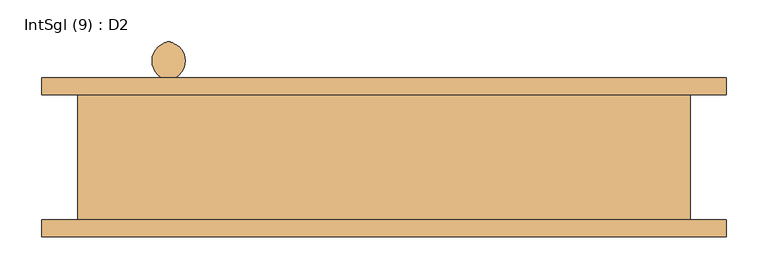
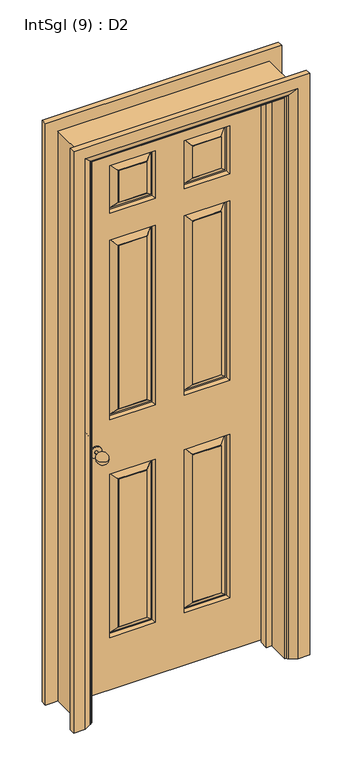
"""IFC4 building model written with IfcOpenShell, lengths in millimetres: door geometry, IntSgl (9) : D2."""

from ifc_helpers import new_model, si_unit, point, frame, origin, place, context, project, spatial, polyline, circle_curve, ellipse_curve, trimmed, outline, extrude, faceted_brep, source, transform, mapped, element, save
from ifc_brep_helpers import plane_surface, cylinder_surface, revolved_surface, advanced_brep


def intsgl_9_d2_8283ee4d(model_context):
    return source(origin(), model_context, "Body", "SolidModel", [
        advanced_brep(
        [(-253.0, 18.0, 900.0), (-258.0, -26.437411, 900.0), (-263.0, 18.0, 900.0), (-263.0, 33.0, 900.0), (-253.0, 33.0, 900.0), (-278.0, 37.0, 900.0), (-238.0, 37.0, 900.0), (-278.0, 33.0, 900.0), (-238.0, 33.0, 900.0)],
        [
            (0, 1, circle_curve(frame((-261.1884862, -3.5786495, 900.0), z_axis=(0.0, 0.0, -1.0), x_axis=(0.0, 1.0, 0.0)), 23.0800654)),
            (1, 2, circle_curve(frame((-254.8115138, -3.5786495, 900.0), z_axis=(0.0, 0.0, -1.0), x_axis=(0.0, 1.0, 0.0)), 23.0800654)),
            (2, 0, circle_curve(frame((-258.0, 18.0, 900.0), z_axis=(0.0, -1.0, 0.0), x_axis=(-1.0, 0.0, 0.0)), 5.0)),
            (0, 2, circle_curve(frame((-258.0, 18.0, 900.0), z_axis=(0.0, -1.0, 0.0), x_axis=(-1.0, 0.0, 0.0)), 5.0)),
            (2, 3),
            (3, 4, circle_curve(frame((-258.0, 33.0, 900.0), z_axis=(0.0, -1.0, 0.0), x_axis=(-1.0, 0.0, 0.0)), 5.0)),
            (4, 0),
            (4, 3, circle_curve(frame((-258.0, 33.0, 900.0), z_axis=(0.0, -1.0, 0.0), x_axis=(-1.0, 0.0, 0.0)), 5.0)),
            (5, 6, circle_curve(frame((-258.0, 37.0, 900.0), z_axis=(0.0, 1.0, 0.0), x_axis=(1.0, 0.0, 0.0)), 20.0)),
            (6, 5, circle_curve(frame((-258.0, 37.0, 900.0), z_axis=(0.0, 1.0, 0.0), x_axis=(1.0, 0.0, 0.0)), 20.0)),
            (7, 8, circle_curve(frame((-258.0, 33.0, 900.0), z_axis=(0.0, -1.0, 0.0), x_axis=(1.0, 0.0, 0.0)), 20.0)),
            (8, 7, circle_curve(frame((-258.0, 33.0, 900.0), z_axis=(0.0, -1.0, 0.0), x_axis=(1.0, 0.0, 0.0)), 20.0)),
            (6, 8),
            (7, 5),
        ],
        [
            revolved_surface(trimmed(ellipse_curve(frame((-254.8115138, -3.5786495, 900.0), z_axis=(0.0, 0.0, -1.0), x_axis=(0.0, 1.0, 0.0)), 23.0800654, 23.0800654), [point((-258.0, -26.437411, 900.0))], [point((-263.0, 18.0, 900.0))], True, "CARTESIAN"), (-258.0, 33.0, 900.0), (0.0, 1.0, 0.0)),
            cylinder_surface(frame((-258.0, 33.0, 900.0), z_axis=(0.0, 1.0, 0.0), x_axis=(-1.0, 0.0, 0.0)), 5.0),
            plane_surface(frame((-238.0, 37.0, 900.0), z_axis=(0.0, 1.0, 0.0), x_axis=(0.0, 0.0, 1.0))),
            plane_surface(frame((-238.0, 33.0, 900.0), z_axis=(0.0, -1.0, 0.0), x_axis=(0.0, 0.0, -1.0))),
            cylinder_surface(frame((-258.0, 33.0, 900.0), z_axis=(0.0, 1.0, 0.0), x_axis=(1.0, 0.0, 0.0)), 20.0),
        ],
        [
            (0, [[1, 2, 3]]),
            (0, [[-1, 4, -2]]),
            (1, [[5, 6, 7, -3]]),
            (1, [[-7, 8, -5, -4]]),
            (2, [[9, 10]]),
            (3, [[11, 12], [-8, -6]]),
            (4, [[13, -11, 14, -10]]),
            (4, [[-14, -12, -13, -9]]),
        ],
    ),
        advanced_brep(
        [(-253.0, 94.0, 900.0), (-263.0, 94.0, 900.0), (-258.0, 138.437411, 900.0), (-253.0, 79.0, 900.0), (-263.0, 79.0, 900.0), (-278.0, 75.0, 900.0), (-238.0, 75.0, 900.0), (-278.0, 79.0, 900.0), (-238.0, 79.0, 900.0)],
        [
            (0, 1, circle_curve(frame((-258.0, 94.0, 900.0), z_axis=(0.0, 1.0, 0.0), x_axis=(-1.0, 0.0, 0.0)), 5.0)),
            (1, 2, circle_curve(frame((-254.8115138, 115.5786495, 900.0), z_axis=(0.0, 0.0, -1.0), x_axis=(0.0, -1.0, 0.0)), 23.0800654)),
            (2, 0, circle_curve(frame((-261.1884862, 115.5786495, 900.0), z_axis=(0.0, 0.0, -1.0), x_axis=(0.0, -1.0, 0.0)), 23.0800654)),
            (1, 0, circle_curve(frame((-258.0, 94.0, 900.0), z_axis=(0.0, 1.0, 0.0), x_axis=(-1.0, 0.0, 0.0)), 5.0)),
            (0, 3),
            (3, 4, circle_curve(frame((-258.0, 79.0, 900.0), z_axis=(0.0, 1.0, 0.0), x_axis=(-1.0, 0.0, 0.0)), 5.0)),
            (4, 1),
            (4, 3, circle_curve(frame((-258.0, 79.0, 900.0), z_axis=(0.0, 1.0, 0.0), x_axis=(-1.0, 0.0, 0.0)), 5.0)),
            (5, 6, circle_curve(frame((-258.0, 75.0, 900.0), z_axis=(0.0, -1.0, 0.0), x_axis=(1.0, 0.0, 0.0)), 20.0)),
            (6, 5, circle_curve(frame((-258.0, 75.0, 900.0), z_axis=(0.0, -1.0, 0.0), x_axis=(1.0, 0.0, 0.0)), 20.0)),
            (7, 8, circle_curve(frame((-258.0, 79.0, 900.0), z_axis=(0.0, 1.0, 0.0), x_axis=(1.0, 0.0, 0.0)), 20.0)),
            (8, 7, circle_curve(frame((-258.0, 79.0, 900.0), z_axis=(0.0, 1.0, 0.0), x_axis=(1.0, 0.0, 0.0)), 20.0)),
            (5, 7),
            (8, 6),
        ],
        [
            revolved_surface(trimmed(ellipse_curve(frame((-254.8115138, 115.5786495, 900.0), z_axis=(0.0, 0.0, 1.0), x_axis=(0.0, -1.0, 0.0)), 23.0800654, 23.0800654), [point((-258.0, 138.437411, 900.0))], [point((-263.0, 94.0, 900.0))], True, "CARTESIAN"), (-258.0, 79.0, 900.0), (0.0, -1.0, 0.0)),
            cylinder_surface(frame((-258.0, 79.0, 900.0), z_axis=(0.0, -1.0, 0.0), x_axis=(-1.0, 0.0, 0.0)), 5.0),
            plane_surface(frame((-238.0, 75.0, 900.0), z_axis=(0.0, -1.0, 0.0), x_axis=(0.0, 0.0, 1.0))),
            plane_surface(frame((-238.0, 79.0, 900.0), z_axis=(0.0, 1.0, 0.0), x_axis=(0.0, 0.0, -1.0))),
            cylinder_surface(frame((-258.0, 79.0, 900.0), z_axis=(0.0, -1.0, 0.0), x_axis=(1.0, 0.0, 0.0)), 20.0),
        ],
        [
            (0, [[1, 2, 3]]),
            (0, [[-2, 4, -3]]),
            (1, [[-1, 5, 6, 7]]),
            (1, [[-4, -7, 8, -5]]),
            (2, [[9, 10]]),
            (3, [[11, 12], [-6, -8]]),
            (4, [[-9, 13, -12, 14]]),
            (4, [[-10, -14, -11, -13]]),
        ],
    ),
        faceted_brep([(-333.0, 37.0, 2058.0), (-333.0, 37.0, 8.0), (333.0, 37.0, 8.0), (333.0, 37.0, 2058.0), (-50.0, 37.0, 800.0), (-50.0, 37.0, 200.0), (-208.0, 37.0, 200.0), (-208.0, 37.0, 800.0), (208.0, 37.0, 800.0), (208.0, 37.0, 200.0), (50.0, 37.0, 200.0), (50.0, 37.0, 800.0), (-50.0, 37.0, 1658.0), (-50.0, 37.0, 1000.0), (-208.0, 37.0, 1000.0), (-208.0, 37.0, 1658.0), (208.0, 37.0, 1658.0), (208.0, 37.0, 1000.0), (50.0, 37.0, 1000.0), (50.0, 37.0, 1658.0), (-50.0, 37.0, 1933.0), (-50.0, 37.0, 1758.0), (-208.0, 37.0, 1758.0), (-208.0, 37.0, 1933.0), (208.0, 37.0, 1933.0), (208.0, 37.0, 1758.0), (50.0, 37.0, 1758.0), (50.0, 37.0, 1933.0), (-80.0, 37.0, 230.0), (-80.0, 37.0, 770.0), (-178.0, 37.0, 770.0), (-178.0, 37.0, 230.0), (178.0, 37.0, 230.0), (178.0, 37.0, 770.0), (80.0, 37.0, 770.0), (80.0, 37.0, 230.0), (-80.0, 37.0, 1030.0), (-80.0, 37.0, 1628.0), (-178.0, 37.0, 1628.0), (-178.0, 37.0, 1030.0), (178.0, 37.0, 1030.0), (178.0, 37.0, 1628.0), (80.0, 37.0, 1628.0), (80.0, 37.0, 1030.0), (-80.0, 37.0, 1788.0), (-80.0, 37.0, 1903.0), (-178.0, 37.0, 1903.0), (-178.0, 37.0, 1788.0), (178.0, 37.0, 1788.0), (178.0, 37.0, 1903.0), (80.0, 37.0, 1903.0), (80.0, 37.0, 1788.0), (-333.0, 75.0, 2058.0), (333.0, 75.0, 2058.0), (333.0, 75.0, 8.0), (-333.0, 75.0, 8.0), (50.0, 75.0, 800.0), (50.0, 75.0, 200.0), (208.0, 75.0, 200.0), (208.0, 75.0, 800.0), (-208.0, 75.0, 800.0), (-208.0, 75.0, 200.0), (-50.0, 75.0, 200.0), (-50.0, 75.0, 800.0), (50.0, 75.0, 1658.0), (50.0, 75.0, 1000.0), (208.0, 75.0, 1000.0), (208.0, 75.0, 1658.0), (-208.0, 75.0, 1658.0), (-208.0, 75.0, 1000.0), (-50.0, 75.0, 1000.0), (-50.0, 75.0, 1658.0), (50.0, 75.0, 1933.0), (50.0, 75.0, 1758.0), (208.0, 75.0, 1758.0), (208.0, 75.0, 1933.0), (-208.0, 75.0, 1933.0), (-208.0, 75.0, 1758.0), (-50.0, 75.0, 1758.0), (-50.0, 75.0, 1933.0), (80.0, 75.0, 230.0), (80.0, 75.0, 770.0), (178.0, 75.0, 770.0), (178.0, 75.0, 230.0), (-178.0, 75.0, 230.0), (-178.0, 75.0, 770.0), (-80.0, 75.0, 770.0), (-80.0, 75.0, 230.0), (80.0, 75.0, 1030.0), (80.0, 75.0, 1628.0), (178.0, 75.0, 1628.0), (178.0, 75.0, 1030.0), (-178.0, 75.0, 1030.0), (-178.0, 75.0, 1628.0), (-80.0, 75.0, 1628.0), (-80.0, 75.0, 1030.0), (80.0, 75.0, 1788.0), (80.0, 75.0, 1903.0), (178.0, 75.0, 1903.0), (178.0, 75.0, 1788.0), (-178.0, 75.0, 1788.0), (-178.0, 75.0, 1903.0), (-80.0, 75.0, 1903.0), (-80.0, 75.0, 1788.0), (80.0, 74.0, 230.0), (80.0, 74.0, 770.0), (58.0, 60.0, 208.0), (58.0, 60.0, 792.0), (78.0, 74.0, 772.0), (78.0, 74.0, 228.0), (53.0, 60.0, 797.0), (53.0, 60.0, 203.0), (178.0, 74.0, 770.0), (200.0, 60.0, 792.0), (180.0, 74.0, 772.0), (205.0, 60.0, 797.0), (178.0, 74.0, 230.0), (200.0, 60.0, 208.0), (180.0, 74.0, 228.0), (205.0, 60.0, 203.0), (-178.0, 74.0, 230.0), (-178.0, 74.0, 770.0), (-200.0, 60.0, 208.0), (-200.0, 60.0, 792.0), (-180.0, 74.0, 772.0), (-180.0, 74.0, 228.0), (-205.0, 60.0, 797.0), (-205.0, 60.0, 203.0), (-80.0, 74.0, 770.0), (-58.0, 60.0, 792.0), (-78.0, 74.0, 772.0), (-53.0, 60.0, 797.0), (-80.0, 74.0, 230.0), (-58.0, 60.0, 208.0), (-78.0, 74.0, 228.0), (-53.0, 60.0, 203.0), (80.0, 74.0, 1030.0), (80.0, 74.0, 1628.0), (58.0, 60.0, 1008.0), (58.0, 60.0, 1650.0), (78.0, 74.0, 1630.0), (78.0, 74.0, 1028.0), (53.0, 60.0, 1655.0), (53.0, 60.0, 1003.0), (178.0, 74.0, 1628.0), (200.0, 60.0, 1650.0), (180.0, 74.0, 1630.0), (205.0, 60.0, 1655.0), (178.0, 74.0, 1030.0), (200.0, 60.0, 1008.0), (180.0, 74.0, 1028.0), (205.0, 60.0, 1003.0), (-178.0, 74.0, 1030.0), (-178.0, 74.0, 1628.0), (-200.0, 60.0, 1008.0), (-200.0, 60.0, 1650.0), (-180.0, 74.0, 1630.0), (-180.0, 74.0, 1028.0), (-205.0, 60.0, 1655.0), (-205.0, 60.0, 1003.0), (-80.0, 74.0, 1628.0), (-58.0, 60.0, 1650.0), (-78.0, 74.0, 1630.0), (-53.0, 60.0, 1655.0), (-80.0, 74.0, 1030.0), (-58.0, 60.0, 1008.0), (-78.0, 74.0, 1028.0), (-53.0, 60.0, 1003.0), (80.0, 74.0, 1788.0), (80.0, 74.0, 1903.0), (58.0, 60.0, 1766.0), (58.0, 60.0, 1925.0), (78.0, 74.0, 1905.0), (78.0, 74.0, 1786.0), (53.0, 60.0, 1930.0), (53.0, 60.0, 1761.0), (178.0, 74.0, 1903.0), (200.0, 60.0, 1925.0), (180.0, 74.0, 1905.0), (205.0, 60.0, 1930.0), (178.0, 74.0, 1788.0), (200.0, 60.0, 1766.0), (180.0, 74.0, 1786.0), (205.0, 60.0, 1761.0), (-178.0, 74.0, 1788.0), (-178.0, 74.0, 1903.0), (-200.0, 60.0, 1766.0), (-200.0, 60.0, 1925.0), (-180.0, 74.0, 1905.0), (-180.0, 74.0, 1786.0), (-205.0, 60.0, 1930.0), (-205.0, 60.0, 1761.0), (-80.0, 74.0, 1903.0), (-58.0, 60.0, 1925.0), (-78.0, 74.0, 1905.0), (-53.0, 60.0, 1930.0), (-80.0, 74.0, 1788.0), (-58.0, 60.0, 1766.0), (-78.0, 74.0, 1786.0), (-53.0, 60.0, 1761.0), (-80.0, 38.0, 230.0), (-80.0, 38.0, 770.0), (-58.0, 52.0, 208.0), (-58.0, 52.0, 792.0), (-78.0, 38.0, 772.0), (-78.0, 38.0, 228.0), (-53.0, 52.0, 797.0), (-53.0, 52.0, 203.0), (-178.0, 38.0, 770.0), (-200.0, 52.0, 792.0), (-180.0, 38.0, 772.0), (-205.0, 52.0, 797.0), (-178.0, 38.0, 230.0), (-200.0, 52.0, 208.0), (-180.0, 38.0, 228.0), (-205.0, 52.0, 203.0), (178.0, 38.0, 230.0), (178.0, 38.0, 770.0), (200.0, 52.0, 208.0), (200.0, 52.0, 792.0), (180.0, 38.0, 772.0), (180.0, 38.0, 228.0), (205.0, 52.0, 797.0), (205.0, 52.0, 203.0), (80.0, 38.0, 770.0), (58.0, 52.0, 792.0), (78.0, 38.0, 772.0), (53.0, 52.0, 797.0), (80.0, 38.0, 230.0), (58.0, 52.0, 208.0), (78.0, 38.0, 228.0), (53.0, 52.0, 203.0), (-80.0, 38.0, 1030.0), (-80.0, 38.0, 1628.0), (-58.0, 52.0, 1008.0), (-58.0, 52.0, 1650.0), (-78.0, 38.0, 1630.0), (-78.0, 38.0, 1028.0), (-53.0, 52.0, 1655.0), (-53.0, 52.0, 1003.0), (-178.0, 38.0, 1628.0), (-200.0, 52.0, 1650.0), (-180.0, 38.0, 1630.0), (-205.0, 52.0, 1655.0), (-178.0, 38.0, 1030.0), (-200.0, 52.0, 1008.0), (-180.0, 38.0, 1028.0), (-205.0, 52.0, 1003.0), (178.0, 38.0, 1030.0), (178.0, 38.0, 1628.0), (200.0, 52.0, 1008.0), (200.0, 52.0, 1650.0), (180.0, 38.0, 1630.0), (180.0, 38.0, 1028.0), (205.0, 52.0, 1655.0), (205.0, 52.0, 1003.0), (80.0, 38.0, 1628.0), (58.0, 52.0, 1650.0), (78.0, 38.0, 1630.0), (53.0, 52.0, 1655.0), (80.0, 38.0, 1030.0), (58.0, 52.0, 1008.0), (78.0, 38.0, 1028.0), (53.0, 52.0, 1003.0), (-80.0, 38.0, 1788.0), (-80.0, 38.0, 1903.0), (-58.0, 52.0, 1766.0), (-58.0, 52.0, 1925.0), (-78.0, 38.0, 1905.0), (-78.0, 38.0, 1786.0), (-53.0, 52.0, 1930.0), (-53.0, 52.0, 1761.0), (-178.0, 38.0, 1903.0), (-200.0, 52.0, 1925.0), (-180.0, 38.0, 1905.0), (-205.0, 52.0, 1930.0), (-178.0, 38.0, 1788.0), (-200.0, 52.0, 1766.0), (-180.0, 38.0, 1786.0), (-205.0, 52.0, 1761.0), (178.0, 38.0, 1788.0), (178.0, 38.0, 1903.0), (200.0, 52.0, 1766.0), (200.0, 52.0, 1925.0), (180.0, 38.0, 1905.0), (180.0, 38.0, 1786.0), (205.0, 52.0, 1930.0), (205.0, 52.0, 1761.0), (80.0, 38.0, 1903.0), (58.0, 52.0, 1925.0), (78.0, 38.0, 1905.0), (53.0, 52.0, 1930.0), (80.0, 38.0, 1788.0), (58.0, 52.0, 1766.0), (78.0, 38.0, 1786.0), (53.0, 52.0, 1761.0)], [[[0, 1, 2, 3], [4, 5, 6, 7], [8, 9, 10, 11], [12, 13, 14, 15], [16, 17, 18, 19], [20, 21, 22, 23], [24, 25, 26, 27]], [[28, 29, 30, 31]], [[32, 33, 34, 35]], [[36, 37, 38, 39]], [[40, 41, 42, 43]], [[44, 45, 46, 47]], [[48, 49, 50, 51]], [[52, 53, 54, 55], [56, 57, 58, 59], [60, 61, 62, 63], [64, 65, 66, 67], [68, 69, 70, 71], [72, 73, 74, 75], [76, 77, 78, 79]], [[80, 81, 82, 83]], [[84, 85, 86, 87]], [[88, 89, 90, 91]], [[92, 93, 94, 95]], [[96, 97, 98, 99]], [[100, 101, 102, 103]], [[1, 0, 52, 55]], [[2, 1, 55, 54]], [[3, 2, 54, 53]], [[0, 3, 53, 52]], [[104, 105, 81, 80]], [[106, 107, 108, 109]], [[56, 110, 111, 57]], [[81, 105, 112, 82]], [[108, 107, 113, 114]], [[110, 56, 59, 115]], [[82, 112, 116, 83]], [[114, 113, 117, 118]], [[115, 59, 58, 119]], [[104, 80, 83, 116]], [[109, 108, 114, 118], [105, 104, 116, 112]], [[106, 109, 118, 117]], [[111, 110, 115, 119], [107, 106, 117, 113]], [[57, 111, 119, 58]], [[120, 121, 85, 84]], [[122, 123, 124, 125]], [[60, 126, 127, 61]], [[85, 121, 128, 86]], [[124, 123, 129, 130]], [[126, 60, 63, 131]], [[86, 128, 132, 87]], [[130, 129, 133, 134]], [[131, 63, 62, 135]], [[120, 84, 87, 132]], [[125, 124, 130, 134], [121, 120, 132, 128]], [[122, 125, 134, 133]], [[127, 126, 131, 135], [123, 122, 133, 129]], [[61, 127, 135, 62]], [[136, 137, 89, 88]], [[138, 139, 140, 141]], [[64, 142, 143, 65]], [[89, 137, 144, 90]], [[140, 139, 145, 146]], [[142, 64, 67, 147]], [[90, 144, 148, 91]], [[146, 145, 149, 150]], [[147, 67, 66, 151]], [[136, 88, 91, 148]], [[141, 140, 146, 150], [137, 136, 148, 144]], [[138, 141, 150, 149]], [[143, 142, 147, 151], [139, 138, 149, 145]], [[65, 143, 151, 66]], [[152, 153, 93, 92]], [[154, 155, 156, 157]], [[68, 158, 159, 69]], [[93, 153, 160, 94]], [[156, 155, 161, 162]], [[158, 68, 71, 163]], [[94, 160, 164, 95]], [[162, 161, 165, 166]], [[163, 71, 70, 167]], [[152, 92, 95, 164]], [[157, 156, 162, 166], [153, 152, 164, 160]], [[154, 157, 166, 165]], [[159, 158, 163, 167], [155, 154, 165, 161]], [[69, 159, 167, 70]], [[168, 169, 97, 96]], [[170, 171, 172, 173]], [[72, 174, 175, 73]], [[97, 169, 176, 98]], [[172, 171, 177, 178]], [[174, 72, 75, 179]], [[98, 176, 180, 99]], [[178, 177, 181, 182]], [[179, 75, 74, 183]], [[168, 96, 99, 180]], [[173, 172, 178, 182], [169, 168, 180, 176]], [[170, 173, 182, 181]], [[175, 174, 179, 183], [171, 170, 181, 177]], [[73, 175, 183, 74]], [[184, 185, 101, 100]], [[186, 187, 188, 189]], [[76, 190, 191, 77]], [[101, 185, 192, 102]], [[188, 187, 193, 194]], [[190, 76, 79, 195]], [[102, 192, 196, 103]], [[194, 193, 197, 198]], [[195, 79, 78, 199]], [[184, 100, 103, 196]], [[189, 188, 194, 198], [185, 184, 196, 192]], [[186, 189, 198, 197]], [[191, 190, 195, 199], [187, 186, 197, 193]], [[77, 191, 199, 78]], [[200, 201, 29, 28]], [[202, 203, 204, 205]], [[4, 206, 207, 5]], [[29, 201, 208, 30]], [[204, 203, 209, 210]], [[206, 4, 7, 211]], [[30, 208, 212, 31]], [[210, 209, 213, 214]], [[211, 7, 6, 215]], [[200, 28, 31, 212]], [[205, 204, 210, 214], [201, 200, 212, 208]], [[202, 205, 214, 213]], [[207, 206, 211, 215], [203, 202, 213, 209]], [[5, 207, 215, 6]], [[216, 217, 33, 32]], [[218, 219, 220, 221]], [[8, 222, 223, 9]], [[33, 217, 224, 34]], [[220, 219, 225, 226]], [[222, 8, 11, 227]], [[34, 224, 228, 35]], [[226, 225, 229, 230]], [[227, 11, 10, 231]], [[216, 32, 35, 228]], [[221, 220, 226, 230], [217, 216, 228, 224]], [[218, 221, 230, 229]], [[223, 222, 227, 231], [219, 218, 229, 225]], [[9, 223, 231, 10]], [[232, 233, 37, 36]], [[234, 235, 236, 237]], [[12, 238, 239, 13]], [[37, 233, 240, 38]], [[236, 235, 241, 242]], [[238, 12, 15, 243]], [[38, 240, 244, 39]], [[242, 241, 245, 246]], [[243, 15, 14, 247]], [[232, 36, 39, 244]], [[237, 236, 242, 246], [233, 232, 244, 240]], [[234, 237, 246, 245]], [[239, 238, 243, 247], [235, 234, 245, 241]], [[13, 239, 247, 14]], [[248, 249, 41, 40]], [[250, 251, 252, 253]], [[16, 254, 255, 17]], [[41, 249, 256, 42]], [[252, 251, 257, 258]], [[254, 16, 19, 259]], [[42, 256, 260, 43]], [[258, 257, 261, 262]], [[259, 19, 18, 263]], [[248, 40, 43, 260]], [[253, 252, 258, 262], [249, 248, 260, 256]], [[250, 253, 262, 261]], [[255, 254, 259, 263], [251, 250, 261, 257]], [[17, 255, 263, 18]], [[264, 265, 45, 44]], [[266, 267, 268, 269]], [[20, 270, 271, 21]], [[45, 265, 272, 46]], [[268, 267, 273, 274]], [[270, 20, 23, 275]], [[46, 272, 276, 47]], [[274, 273, 277, 278]], [[275, 23, 22, 279]], [[264, 44, 47, 276]], [[269, 268, 274, 278], [265, 264, 276, 272]], [[266, 269, 278, 277]], [[271, 270, 275, 279], [267, 266, 277, 273]], [[21, 271, 279, 22]], [[280, 281, 49, 48]], [[282, 283, 284, 285]], [[24, 286, 287, 25]], [[49, 281, 288, 50]], [[284, 283, 289, 290]], [[286, 24, 27, 291]], [[50, 288, 292, 51]], [[290, 289, 293, 294]], [[291, 27, 26, 295]], [[280, 48, 51, 292]], [[285, 284, 290, 294], [281, 280, 292, 288]], [[282, 285, 294, 293]], [[287, 286, 291, 295], [283, 282, 293, 289]], [[25, 287, 295, 26]]]),
        faceted_brep([(-335.0, 75.0, 0.0), (-335.0, -75.0, 0.0), (-367.0, -75.0, 0.0), (-367.0, 75.0, 0.0), (-335.0, 75.0, 2060.0), (-335.0, -75.0, 2060.0), (-367.0, -75.0, 2092.0), (-367.0, 75.0, 2092.0), (335.0, 75.0, 0.0), (367.0, 75.0, 0.0), (367.0, -75.0, 0.0), (335.0, -75.0, 0.0), (335.0, 75.0, 2060.0), (367.0, 75.0, 2092.0), (367.0, -75.0, 2092.0), (335.0, -75.0, 2060.0)], [[[0, 1, 2, 3]], [[1, 0, 4, 5]], [[2, 1, 5, 6]], [[3, 2, 6, 7]], [[0, 3, 7, 4]], [[8, 9, 10, 11]], [[12, 13, 9, 8]], [[13, 14, 10, 9]], [[14, 15, 11, 10]], [[15, 12, 8, 11]], [[5, 4, 12, 15]], [[6, 5, 15, 14]], [[7, 6, 14, 13]], [[4, 7, 13, 12]]]),
        extrude(outline(polyline([(0.0, -335.0), (0.0, -316.0), (2041.0, -316.0), (2041.0, 316.0), (0.0, 316.0), (0.0, 335.0), (2060.0, 335.0), (2060.0, -335.0), (0.0, -335.0)])), frame((0.0, 3.0, 0.0), z_axis=(0.0, 1.0, 0.0), x_axis=(0.0, 0.0, 1.0)), (0.0, 0.0, 1.0), 32.0),
        advanced_brep(
        [(-410.0, -95.0, 0.0), (-410.0, -75.0, 0.0), (-340.0, -75.0, 0.0), (-344.0, -81.0, 0.0), (-370.0, -95.0, 0.0), (-410.0, -95.0, 2135.0), (-410.0, -75.0, 2135.0), (410.0, -75.0, 2135.0), (410.0, -75.0, 0.0), (340.0, -75.0, 0.0), (340.0, -75.0, 2065.0), (-340.0, -75.0, 2065.0), (-344.0, -81.0, 2069.0), (-370.0, -95.0, 2095.0), (370.0, -95.0, 2095.0), (370.0, -95.0, 0.0), (410.0, -95.0, 0.0), (410.0, -95.0, 2135.0), (344.0, -81.0, 0.0), (344.0, -81.0, 2069.0)],
        [
            (0, 1),
            (1, 2),
            (2, 3, circle_curve(frame((-348.0, -74.0, 0.0), z_axis=(0.0, 0.0, -1.0), x_axis=(-1.0, 0.0, 0.0)), 8.0622577)),
            (3, 4),
            (4, 0),
            (0, 5),
            (5, 6),
            (6, 1),
            (6, 7),
            (7, 8),
            (8, 9),
            (9, 10),
            (10, 11),
            (11, 2),
            (11, 12, ellipse_curve(frame((-348.0, -74.0, 2073.0), z_axis=(-0.7071067811865475, 0.0, -0.7071067811865475), x_axis=(0.7071067811865474, 0.0, -0.7071067811865476)), 11.4017543, 8.0622577)),
            (12, 3),
            (12, 13),
            (13, 4),
            (13, 14),
            (14, 15),
            (15, 16),
            (16, 17),
            (17, 5),
            (7, 17),
            (16, 8),
            (15, 18),
            (18, 9, circle_curve(frame((348.0, -74.0, 0.0), z_axis=(0.0, 0.0, -1.0), x_axis=(1.0, 0.0, 0.0)), 8.0622577)),
            (19, 10, ellipse_curve(frame((348.0, -74.0, 2073.0), z_axis=(0.7071067811865475, 0.0, -0.7071067811865475), x_axis=(0.7071067811865474, 0.0, 0.7071067811865476)), 11.4017543, 8.0622577)),
            (18, 19),
            (14, 19),
            (19, 12),
        ],
        [
            plane_surface(frame((-340.0, -75.0, 0.0), z_axis=(0.0, 0.0, -1.0), x_axis=(0.0, -1.0, 0.0))),
            plane_surface(frame((-410.0, -95.0, 0.0), z_axis=(-1.0, 0.0, 0.0), x_axis=(0.0, 0.0, 1.0))),
            plane_surface(frame((-410.0, -75.0, 0.0), z_axis=(0.0, 1.0, 0.0), x_axis=(0.0, 0.0, 1.0))),
            cylinder_surface(frame((-348.0, -74.0, 0.0), z_axis=(0.0, 0.0, -1.0), x_axis=(-1.0, 0.0, 0.0)), 8.0622577),
            plane_surface(frame((-344.0, -81.0, 0.0), z_axis=(0.4740998230350183, -0.8804710999221749, 0.0), x_axis=(0.0, 0.0, 1.0))),
            plane_surface(frame((-370.0, -95.0, 0.0), z_axis=(0.0, -1.0, 0.0), x_axis=(0.0, 0.0, 1.0))),
            plane_surface(frame((410.0, -95.0, 2135.0), z_axis=(1.0, 0.0, 0.0), x_axis=(0.0, 0.0, -1.0))),
            plane_surface(frame((340.0, -75.0, 0.0), z_axis=(0.0, 0.0, -1.0), x_axis=(0.0, -1.0, 0.0))),
            cylinder_surface(frame((348.0, -74.0, 2065.0), z_axis=(0.0, 0.0, 1.0), x_axis=(1.0, 0.0, 0.0)), 8.0622577),
            plane_surface(frame((344.0, -81.0, 2069.0), z_axis=(-0.4740998230350183, -0.8804710999221749, 0.0), x_axis=(0.0, 0.0, -1.0))),
            plane_surface(frame((-410.0, -95.0, 2135.0), z_axis=(0.0, 0.0, 1.0), x_axis=(1.0, 0.0, 0.0))),
            cylinder_surface(frame((-340.0, -74.0, 2073.0), z_axis=(-1.0, 0.0, 0.0), x_axis=(0.0, 0.0, 1.0)), 8.0622577),
            plane_surface(frame((-344.0, -81.0, 2069.0), z_axis=(0.0, -0.8804710999221749, -0.4740998230350183), x_axis=(1.0, 0.0, 0.0))),
        ],
        [
            (0, [[1, 2, 3, 4, 5]]),
            (1, [[-1, 6, 7, 8]]),
            (2, [[-2, -8, 9, 10, 11, 12, 13, 14]]),
            (3, [[-3, -14, 15, 16]]),
            (4, [[-4, -16, 17, 18]]),
            (5, [[-5, -18, 19, 20, 21, 22, 23, -6]]),
            (6, [[24, -22, 25, -10]]),
            (7, [[-21, 26, 27, -11, -25]]),
            (8, [[28, -12, -27, 29]]),
            (9, [[30, -29, -26, -20]]),
            (10, [[-7, -23, -24, -9]]),
            (11, [[-15, -13, -28, 31]]),
            (12, [[-17, -31, -30, -19]]),
        ],
    ),
        advanced_brep(
        [(410.0, 95.0, 0.0), (410.0, 75.0, 0.0), (340.0, 75.0, 0.0), (344.0, 81.0, 0.0), (370.0, 95.0, 0.0), (410.0, 95.0, 2135.0), (410.0, 75.0, 2135.0), (-410.0, 75.0, 2135.0), (-410.0, 75.0, 0.0), (-340.0, 75.0, 0.0), (-340.0, 75.0, 2065.0), (340.0, 75.0, 2065.0), (344.0, 81.0, 2069.0), (370.0, 95.0, 2095.0), (-370.0, 95.0, 2095.0), (-370.0, 95.0, 0.0), (-410.0, 95.0, 0.0), (-410.0, 95.0, 2135.0), (-344.0, 81.0, 0.0), (-344.0, 81.0, 2069.0)],
        [
            (0, 1),
            (1, 2),
            (2, 3, circle_curve(frame((348.0, 74.0, 0.0), z_axis=(0.0, 0.0, -1.0), x_axis=(1.0, 0.0, 0.0)), 8.0622577)),
            (3, 4),
            (4, 0),
            (0, 5),
            (5, 6),
            (6, 1),
            (6, 7),
            (7, 8),
            (8, 9),
            (9, 10),
            (10, 11),
            (11, 2),
            (11, 12, ellipse_curve(frame((348.0, 74.0, 2073.0), z_axis=(0.7071067811865475, 0.0, -0.7071067811865475), x_axis=(-0.7071067811865474, 0.0, -0.7071067811865476)), 11.4017543, 8.0622577)),
            (12, 3),
            (12, 13),
            (13, 4),
            (13, 14),
            (14, 15),
            (15, 16),
            (16, 17),
            (17, 5),
            (7, 17),
            (16, 8),
            (15, 18),
            (18, 9, circle_curve(frame((-348.0, 74.0, 0.0), z_axis=(0.0, 0.0, -1.0), x_axis=(-1.0, 0.0, 0.0)), 8.0622577)),
            (19, 10, ellipse_curve(frame((-348.0, 74.0, 2073.0), z_axis=(-0.7071067811865475, 0.0, -0.7071067811865475), x_axis=(-0.7071067811865474, 0.0, 0.7071067811865476)), 11.4017543, 8.0622577)),
            (18, 19),
            (14, 19),
            (19, 12),
        ],
        [
            plane_surface(frame((340.0, 75.0, 0.0), z_axis=(0.0, 0.0, -1.0), x_axis=(0.0, 1.0, 0.0))),
            plane_surface(frame((410.0, 95.0, 0.0), z_axis=(1.0, 0.0, 0.0), x_axis=(0.0, 0.0, 1.0))),
            plane_surface(frame((410.0, 75.0, 0.0), z_axis=(0.0, -1.0, 0.0), x_axis=(0.0, 0.0, 1.0))),
            cylinder_surface(frame((348.0, 74.0, 0.0), z_axis=(0.0, 0.0, -1.0), x_axis=(1.0, 0.0, 0.0)), 8.0622577),
            plane_surface(frame((344.0, 81.0, 0.0), z_axis=(-0.4740998230350183, 0.8804710999221749, 0.0), x_axis=(0.0, 0.0, 1.0))),
            plane_surface(frame((370.0, 95.0, 0.0), z_axis=(0.0, 1.0, 0.0), x_axis=(0.0, 0.0, 1.0))),
            plane_surface(frame((-410.0, 95.0, 2135.0), z_axis=(-1.0, 0.0, 0.0), x_axis=(0.0, 0.0, -1.0))),
            plane_surface(frame((-340.0, 75.0, 0.0), z_axis=(0.0, 0.0, -1.0), x_axis=(0.0, 1.0, 0.0))),
            cylinder_surface(frame((-348.0, 74.0, 2065.0), z_axis=(0.0, 0.0, 1.0), x_axis=(-1.0, 0.0, 0.0)), 8.0622577),
            plane_surface(frame((-344.0, 81.0, 2069.0), z_axis=(0.4740998230350183, 0.8804710999221749, 0.0), x_axis=(0.0, 0.0, -1.0))),
            plane_surface(frame((410.0, 95.0, 2135.0), z_axis=(0.0, 0.0, 1.0), x_axis=(-1.0, 0.0, 0.0))),
            cylinder_surface(frame((340.0, 74.0, 2073.0), z_axis=(1.0, 0.0, 0.0), x_axis=(0.0, 0.0, 1.0)), 8.0622577),
            plane_surface(frame((344.0, 81.0, 2069.0), z_axis=(0.0, 0.8804710999221749, -0.4740998230350183), x_axis=(-1.0, 0.0, 0.0))),
        ],
        [
            (0, [[1, 2, 3, 4, 5]]),
            (1, [[-1, 6, 7, 8]]),
            (2, [[-2, -8, 9, 10, 11, 12, 13, 14]]),
            (3, [[-3, -14, 15, 16]]),
            (4, [[-4, -16, 17, 18]]),
            (5, [[-5, -18, 19, 20, 21, 22, 23, -6]]),
            (6, [[24, -22, 25, -10]]),
            (7, [[-21, 26, 27, -11, -25]]),
            (8, [[28, -12, -27, 29]]),
            (9, [[30, -29, -26, -20]]),
            (10, [[-7, -23, -24, -9]]),
            (11, [[-15, -13, -28, 31]]),
            (12, [[-17, -31, -30, -19]]),
        ],
    ),
    ])


if __name__ == "__main__":
    model = new_model("IFC4")
    model_context = context("Model", 3, world=origin())
    ifc_project = project(units=[si_unit("LENGTHUNIT", "METRE", prefix="MILLI")], contexts=[model_context])
    site = spatial("IfcSite", under=ifc_project)
    building = spatial("IfcBuilding", under=site)
    placement = place(None, origin())
    intsgl_9_d2_shape = intsgl_9_d2_8283ee4d(model_context)
    element("IfcDoor", 1, ObjectType="IntSgl (9) : D2", at=placement, inside=building, context=model_context, shape_type="MappedRepresentation", body=[
        mapped(intsgl_9_d2_shape, transform((0.0, 0.0, 0.0), x_axis=(1.0, 0.0, 0.0), y_axis=(0.0, 1.0, 0.0), z_axis=(0.0, 0.0, 1.0))),
    ])
    save(model, "model.ifc")

# Revit data of these elements
# Type "IntSgl (9) : D2"
#   Type Mark = "50"
#   Operation = "SingleSwingRight"
#   Manufacturer = "Revit"
#   Keynote = "L20"
#   UnderCut = 8 mm
#   Tolerance = 2 mm
#   Thickness = 38 mm
#   Structural Tolerance = 8 mm
#   StopDepth = 32 mm
#   Stop Thickness = 19 mm
#   Stile Top Rail = 125 mm
#   Stile Shutting = 125 mm
#   Stile Muntin Rail = 100 mm
#   Stile Lock Rail = 200 mm
#   Stile Intermediate/Frieze = 100 mm
#   Stile Hanging = 125 mm
#   Stile Bottom Rail = 200 mm
#   Rough Width = 750 mm
#   Rough Height = 2100 mm
#   Height to Top Lock Rail = 1000 mm
#   Handle Z Distance = 900 mm
#   Handle X Distance = 75 mm
#   Frame Thickness = 32 mm
#   Door Panel Width = 666 mm
#   Height = 2100 mm
#   Width = 750 mm
#   Door Panel Thickness = 38 mm
#   Door Panel Offset = 0 mm
#   Door Panel Height = 2050 mm
#   Architrave Setback = 5 mm
#   Vis - Ironmongery = yes
#   Material Ironmongery = Door - Handle
#   Material Frame = Door - Frame/Mullion
#   Material Door = Door - Panel
#   Material Architrave = Door - Architrave
#   Function = (empty or 0)
#   Wall Closure = (empty or 0)
# Element 1 (IfcDoor, "IntSgl (9) : D2")
#   Materials on its faces: "Door - Panel", "Door - Architrave", "Door - Frame/Mullion", "Door - Handle"
# Materials
#   "Door - Handle": colour RGB 0 0 0, transparency 0, Keynote = "P21", Cost = 0, Export to IFC = 0
#   "Door - Frame/Mullion": class "Wood", colour RGB 212 179 113, transparency 0, Keynote = "L20", Cost = 0, Export to IFC = 0
#   "Door - Panel": class "Wood", colour RGB 210 159 95, transparency 0, Keynote = "L20", Cost = 0, Export to IFC = 0
#   "Door - Architrave": class "Wood", colour RGB 154 90 5, transparency 0, Keynote = "P20", Cost = 0, Export to IFC = 0
